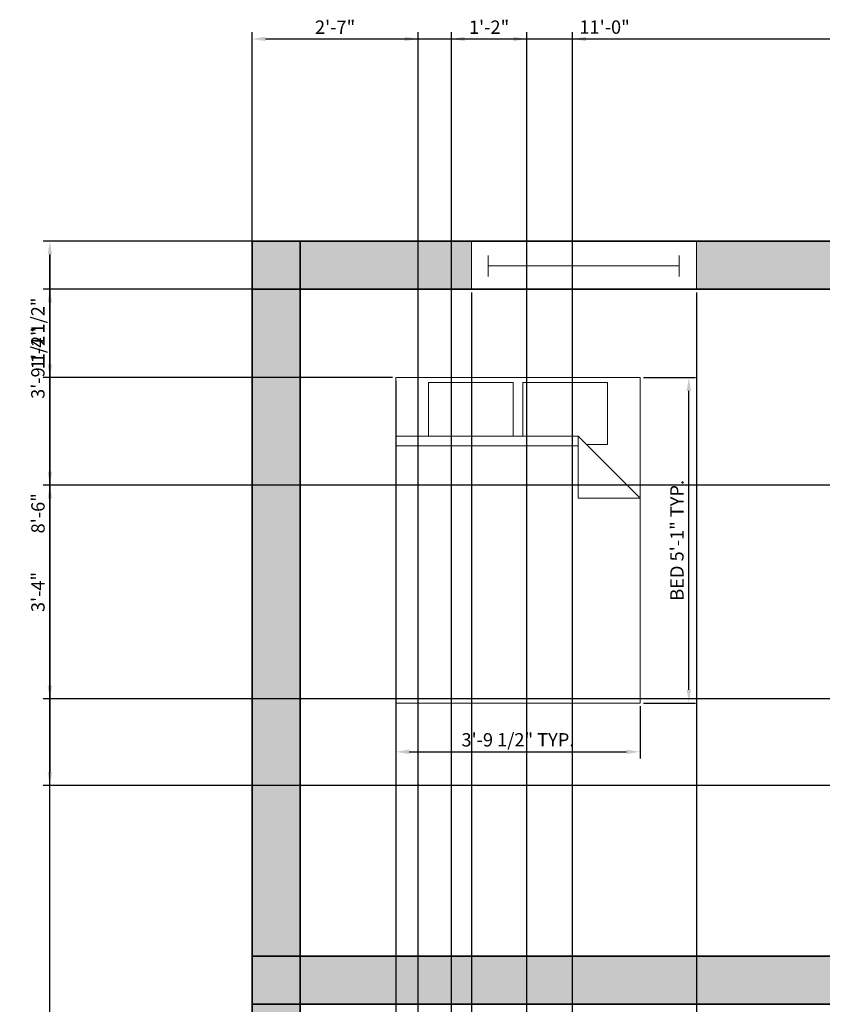
# Model space of a CAD drawing. Units: millimetres. Extents: x 2856 to 3283, y 634 to 1474.
# Tile 4 of 8: x 2856 to 3006, y 1288 to 1472. Entities that reach past the tile are written whole.
import ezdxf

# ---------------------------------------------------------------- set-up
doc = ezdxf.new("R2010")
doc.units = ezdxf.units.MM
for name, color, linetype, lineweight in [('A-ANNO-DIMS', 90, 'Continuous', 18), ('A-WALL-PATT', 2, 'Continuous', 13), ('furniture', 140, 'Continuous', 18), ('walls', 50, 'Continuous', 35), ('windows', 30, 'Continuous', 18)]:
    doc.layers.add(name, color=color, linetype=linetype, lineweight=lineweight)
doc.styles.get("Standard").update_dxf_attribs({"font": 'arial.ttf'})
doc.dimstyles.new('ISO-25', dxfattribs={"dimtxt": 2.5, "dimasz": 2.5, "dimexe": 1.25, "dimexo": 0.625, "dimtad": 1, "dimdec": 0, "dimlunit": 3, "dimtxsty": 'Standard', "dimcen": 2.5, "dimadec": 0, "dimazin": 0, "dimtfac": 1, "dimtdec": 0, "dimtmove": 0, "dimatfit": 3, "dimfxl": 1, "dimarcsym": 0})

# ---------------------------------------------------------------- blocks, each defined once
blk = doc.blocks.new('*U5')
for p, q in [((0, 4), (0, 0)), ((36, 4), (36, 0)), ((0, 2), (36, 2))]:
    blk.add_line(p, q)
blk = doc.blocks.new('Bed - Queen')
for p, q in [((0, -80.00003), (0, 0)), ((0, 0), (59.99999, 0)), ((59.99999, 0), (59.99999, -80.00003)), ((7.99999, -1.2), (28.79998, -1.2)), ((7.99999, -14.4), (7.99999, -1.2)), ((28.79998, -1.2), (28.79998, -14.4)), ((31.19999, -1.2), (51.99999, -1.2)), ((31.19999, -14.4), (31.19999, -1.2)), ((51.99999, -1.2), (51.99999, -16.4)), ((0, -14.4), (44.8, -14.4)), ((59.99999, -29.6), (44.8, -14.4)), ((44.8, -14.4), (44.8, -29.6)), ((44.8, -16.8), (0, -16.8)), ((51.99999, -16.4), (46.79936, -16.4)), ((44.8, -29.6), (59.99999, -29.6)), ((59.99999, -80.00003), (0, -80.00003))]:
    blk.add_line(p, q)
blk = doc.blocks.new('*D16')
at = {"layer": 'A-ANNO-DIMS', "color": 0, "lineweight": -2, "transparency": 16777216}
for p, q in [((2972.43, 1405.35), (2982.2, 1405.35)), ((2980.95, 1346.89), (2980.95, 1402.85)), ((2972.43, 1344.39), (2982.2, 1344.39))]:
    blk.add_line(p, q, dxfattribs=at)
at = {"layer": 'A-ANNO-DIMS', "color": 0, "transparency": 16777216}
for points in [[(2980.53, 1402.85), (2981.36, 1402.85), (2980.95, 1405.35)], [(2980.53, 1346.89), (2981.36, 1346.89), (2980.95, 1344.39)]]:
    blk.add_solid(points, dxfattribs=at)
at = {"layer": 'Defpoints', "color": 0, "transparency": 16777216}
for p in [(2971.8, 1405.35), (2980.95, 1405.35), (2971.8, 1344.39)]:
    blk.add_point(p, dxfattribs=at)
at = {"layer": 'A-ANNO-DIMS', "color": 0, "transparency": 16777216, "insert": (2979.04, 1374.87), "char_height": 2.5, "attachment_point": 5, "rotation": 90}
blk.add_mtext('BED 5\'-1" TYP.', dxfattribs=at)
blk = doc.blocks.new('*D17')
at = {"layer": 'A-ANNO-DIMS', "color": 0, "lineweight": -2, "transparency": 16777216}
for p, q in [((2926.08, 1343.77), (2926.08, 1334)), ((2971.8, 1343.77), (2971.8, 1334)), ((2928.58, 1335.25), (2969.3, 1335.25))]:
    blk.add_line(p, q, dxfattribs=at)
at = {"layer": 'A-ANNO-DIMS', "color": 0, "transparency": 16777216}
for points in [[(2928.58, 1335.66), (2928.58, 1334.83), (2926.08, 1335.25)], [(2969.3, 1335.66), (2969.3, 1334.83), (2971.8, 1335.25)]]:
    blk.add_solid(points, dxfattribs=at)
at = {"layer": 'Defpoints', "color": 0, "transparency": 16777216}
for p in [(2926.08, 1344.39), (2971.8, 1344.39), (2971.8, 1335.25)]:
    blk.add_point(p, dxfattribs=at)
at = {"layer": 'A-ANNO-DIMS', "color": 0, "transparency": 16777216, "insert": (2948.94, 1337.17), "char_height": 2.5, "attachment_point": 5}
blk.add_mtext('3\'-9 1/2" TYP.', dxfattribs=at)
blk = doc.blocks.new('*D29')
at = {"layer": 'A-ANNO-DIMS', "color": 0, "lineweight": -2, "transparency": 16777216}
for p, q in [((2898.55, 1430.94), (2860.05, 1430.94)), ((2861.3, 676.44), (2861.3, 1428.44)), ((2898.55, 673.94), (2860.05, 673.94))]:
    blk.add_line(p, q, dxfattribs=at)
at = {"layer": 'A-ANNO-DIMS', "color": 0, "transparency": 16777216}
for points in [[(2860.88, 1428.44), (2861.72, 1428.44), (2861.3, 1430.94)], [(2860.88, 676.44), (2861.72, 676.44), (2861.3, 673.94)]]:
    blk.add_solid(points, dxfattribs=at)
at = {"layer": 'Defpoints', "color": 0, "transparency": 16777216}
for p in [(2861.3, 1430.94), (2899.17, 1430.94), (2899.17, 673.94)]:
    blk.add_point(p, dxfattribs=at)
at = {"layer": 'A-ANNO-DIMS', "color": 0, "transparency": 16777216, "insert": (2859.4, 1052.44), "char_height": 2.5, "attachment_point": 5, "rotation": 90}
blk.add_mtext('63\'-1"', dxfattribs=at)
blk = doc.blocks.new('*D44')
at = {"layer": 'A-ANNO-DIMS', "color": 0, "lineweight": -2, "transparency": 16777216}
for p, q in [((2899.17, 1431.56), (2899.17, 1470.06)), ((2901.67, 1468.81), (3028.67, 1468.81)), ((3031.17, 1431.56), (3031.17, 1470.06))]:
    blk.add_line(p, q, dxfattribs=at)
at = {"layer": 'A-ANNO-DIMS', "color": 0, "transparency": 16777216}
for points in [[(2901.67, 1469.23), (2901.67, 1468.4), (2899.17, 1468.81)], [(3028.67, 1469.23), (3028.67, 1468.4), (3031.17, 1468.81)]]:
    blk.add_solid(points, dxfattribs=at)
at = {"layer": 'Defpoints', "color": 0, "transparency": 16777216}
for p in [(3031.17, 1468.81), (2899.17, 1430.94), (3031.17, 1430.94)]:
    blk.add_point(p, dxfattribs=at)
at = {"layer": 'A-ANNO-DIMS', "color": 0, "transparency": 16777216, "insert": (2965.17, 1470.71), "char_height": 2.5, "attachment_point": 5}
blk.add_mtext('11\'-0"', dxfattribs=at)
blk = doc.blocks.new('*D48')
at = {"layer": 'A-ANNO-DIMS', "color": 0, "lineweight": -2, "transparency": 16777216}
for p, q in [((3030.55, 1430.94), (2860.05, 1430.94)), ((2861.3, 1428.44), (2861.3, 1331.44)), ((3030.55, 1328.94), (2860.05, 1328.94))]:
    blk.add_line(p, q, dxfattribs=at)
at = {"layer": 'A-ANNO-DIMS', "color": 0, "transparency": 16777216}
for points in [[(2860.88, 1428.44), (2861.72, 1428.44), (2861.3, 1430.94)], [(2860.88, 1331.44), (2861.72, 1331.44), (2861.3, 1328.94)]]:
    blk.add_solid(points, dxfattribs=at)
at = {"layer": 'Defpoints', "color": 0, "transparency": 16777216}
for p in [(3031.17, 1430.94), (2861.3, 1328.94), (3031.17, 1328.94)]:
    blk.add_point(p, dxfattribs=at)
at = {"layer": 'A-ANNO-DIMS', "color": 0, "transparency": 16777216, "insert": (2859.4, 1379.94), "char_height": 2.5, "attachment_point": 5, "rotation": 90}
blk.add_mtext('8\'-6"', dxfattribs=at)
blk = doc.blocks.new('*D59')
at = {"layer": 'A-ANNO-DIMS', "color": 0, "lineweight": -2, "transparency": 16777216}
for p, q in [((2959.17, 1117.56), (2959.17, 1470.06)), ((2961.67, 1468.81), (3071.67, 1468.81)), ((3074.17, 1117.56), (3074.17, 1470.06))]:
    blk.add_line(p, q, dxfattribs=at)
at = {"layer": 'A-ANNO-DIMS', "color": 0, "transparency": 16777216}
for points in [[(2961.67, 1469.23), (2961.67, 1468.4), (2959.17, 1468.81)], [(3071.67, 1469.23), (3071.67, 1468.4), (3074.17, 1468.81)]]:
    blk.add_solid(points, dxfattribs=at)
at = {"layer": 'Defpoints', "color": 0, "transparency": 16777216}
for p in [(3074.17, 1468.81), (2959.17, 1116.94), (3074.17, 1116.94)]:
    blk.add_point(p, dxfattribs=at)
at = {"layer": 'A-ANNO-DIMS', "color": 0, "transparency": 16777216, "insert": (3016.67, 1470.71), "char_height": 2.5, "attachment_point": 5}
blk.add_mtext('9\'-7"', dxfattribs=at)
blk = doc.blocks.new('*D69')
at = {"layer": 'A-ANNO-DIMS', "color": 0, "lineweight": -2, "transparency": 16777216}
for p, q in [((2940.27, 1421.31), (2940.27, 634.81)), ((2982.35, 1421.31), (2982.35, 634.81)), ((2942.77, 636.06), (2979.85, 636.06))]:
    blk.add_line(p, q, dxfattribs=at)
at = {"layer": 'A-ANNO-DIMS', "color": 0, "transparency": 16777216}
for points in [[(2942.77, 636.48), (2942.77, 635.65), (2940.27, 636.06)], [(2979.85, 636.48), (2979.85, 635.65), (2982.35, 636.06)]]:
    blk.add_solid(points, dxfattribs=at)
at = {"layer": 'Defpoints', "color": 0, "transparency": 16777216}
for p in [(2940.27, 1421.94), (2982.35, 1421.94), (2982.35, 636.06)]:
    blk.add_point(p, dxfattribs=at)
at = {"layer": 'A-ANNO-DIMS', "color": 0, "transparency": 16777216, "insert": (2961.31, 637.97), "char_height": 2.5, "attachment_point": 5}
blk.add_mtext('3\'-6"', dxfattribs=at)
blk = doc.blocks.new('*D72')
at = {"layer": 'A-ANNO-DIMS', "color": 0, "lineweight": -2, "transparency": 16777216}
for p, q in [((3233.55, 1385.21), (2860.05, 1385.21)), ((2861.3, 1347.66), (2861.3, 1382.71)), ((3233.55, 1345.16), (2860.05, 1345.16))]:
    blk.add_line(p, q, dxfattribs=at)
at = {"layer": 'A-ANNO-DIMS', "color": 0, "transparency": 16777216}
for points in [[(2860.88, 1382.71), (2861.72, 1382.71), (2861.3, 1385.21)], [(2860.88, 1347.66), (2861.72, 1347.66), (2861.3, 1345.16)]]:
    blk.add_solid(points, dxfattribs=at)
at = {"layer": 'Defpoints', "color": 0, "transparency": 16777216}
for p in [(2861.3, 1385.21), (3234.17, 1385.21), (3234.17, 1345.16)]:
    blk.add_point(p, dxfattribs=at)
at = {"layer": 'A-ANNO-DIMS', "color": 0, "transparency": 16777216, "insert": (2859.4, 1365.19), "char_height": 2.5, "attachment_point": 5, "rotation": 90}
blk.add_mtext('3\'-4"', dxfattribs=at)
blk = doc.blocks.new('*D76')
at = {"layer": 'A-ANNO-DIMS', "color": 0, "lineweight": -2, "transparency": 16777216}
for p, q in [((2899.17, 1421.31), (2899.17, 634.81)), ((2940.27, 1421.31), (2940.27, 634.81)), ((2901.67, 636.06), (2937.77, 636.06))]:
    blk.add_line(p, q, dxfattribs=at)
at = {"layer": 'A-ANNO-DIMS', "color": 0, "transparency": 16777216}
for points in [[(2901.67, 636.48), (2901.67, 635.65), (2899.17, 636.06)], [(2937.77, 636.48), (2937.77, 635.65), (2940.27, 636.06)]]:
    blk.add_solid(points, dxfattribs=at)
at = {"layer": 'Defpoints', "color": 0, "transparency": 16777216}
for p in [(2899.17, 1421.94), (2940.27, 1421.94), (2940.27, 636.06)]:
    blk.add_point(p, dxfattribs=at)
at = {"layer": 'A-ANNO-DIMS', "color": 0, "transparency": 16777216, "insert": (2919.72, 637.97), "char_height": 2.5, "attachment_point": 5}
blk.add_mtext('3\'-5"', dxfattribs=at)
blk = doc.blocks.new('*D78')
at = {"layer": 'A-ANNO-DIMS', "color": 0, "lineweight": -2, "transparency": 16777216}
for p, q in [((3233.55, 1430.94), (2860.05, 1430.94)), ((2861.3, 1387.71), (2861.3, 1428.44)), ((3233.55, 1385.21), (2860.05, 1385.21))]:
    blk.add_line(p, q, dxfattribs=at)
at = {"layer": 'A-ANNO-DIMS', "color": 0, "transparency": 16777216}
for points in [[(2860.88, 1428.44), (2861.72, 1428.44), (2861.3, 1430.94)], [(2860.88, 1387.71), (2861.72, 1387.71), (2861.3, 1385.21)]]:
    blk.add_solid(points, dxfattribs=at)
at = {"layer": 'Defpoints', "color": 0, "transparency": 16777216}
for p in [(2861.3, 1430.94), (3234.17, 1430.94), (3234.17, 1385.21)]:
    blk.add_point(p, dxfattribs=at)
at = {"layer": 'A-ANNO-DIMS', "color": 0, "transparency": 16777216, "insert": (2859.38, 1408.08), "char_height": 2.5, "attachment_point": 5, "rotation": 90}
blk.add_mtext('3\'-9 1/2"', dxfattribs=at)
blk = doc.blocks.new('*D82')
at = {"layer": 'A-ANNO-DIMS', "color": 0, "lineweight": -2, "transparency": 16777216}
for p, q in [((2936.5, 1173.36), (2936.5, 1470.06)), ((2939, 1468.81), (2948.08, 1468.81)), ((2950.58, 1173.36), (2950.58, 1470.06))]:
    blk.add_line(p, q, dxfattribs=at)
at = {"layer": 'A-ANNO-DIMS', "color": 0, "transparency": 16777216}
for points in [[(2939, 1469.23), (2939, 1468.4), (2936.5, 1468.81)], [(2948.08, 1469.23), (2948.08, 1468.4), (2950.58, 1468.81)]]:
    blk.add_solid(points, dxfattribs=at)
at = {"layer": 'Defpoints', "color": 0, "transparency": 16777216}
for p in [(2950.58, 1468.81), (2936.5, 1172.73), (2950.58, 1172.73)]:
    blk.add_point(p, dxfattribs=at)
at = {"layer": 'A-ANNO-DIMS', "color": 0, "transparency": 16777216, "insert": (2943.54, 1470.69), "char_height": 2.5, "attachment_point": 5}
blk.add_mtext('1\'-2"', dxfattribs=at)
blk = doc.blocks.new('*D86')
at = {"layer": 'A-ANNO-DIMS', "color": 0, "lineweight": -2, "transparency": 16777216}
for p, q in [((2899.17, 1059.56), (2899.17, 1470.06)), ((2901.67, 1468.81), (2927.75, 1468.81)), ((2930.25, 1059.56), (2930.25, 1470.06))]:
    blk.add_line(p, q, dxfattribs=at)
at = {"layer": 'A-ANNO-DIMS', "color": 0, "transparency": 16777216}
for points in [[(2901.67, 1469.23), (2901.67, 1468.4), (2899.17, 1468.81)], [(2927.75, 1469.23), (2927.75, 1468.4), (2930.25, 1468.81)]]:
    blk.add_solid(points, dxfattribs=at)
at = {"layer": 'Defpoints', "color": 0, "transparency": 16777216}
for p in [(2930.25, 1468.81), (2899.17, 1058.94), (2930.25, 1058.94)]:
    blk.add_point(p, dxfattribs=at)
at = {"layer": 'A-ANNO-DIMS', "color": 0, "transparency": 16777216, "insert": (2914.71, 1470.69), "char_height": 2.5, "attachment_point": 5}
blk.add_mtext('2\'-7"', dxfattribs=at)
blk = doc.blocks.new('*D90')
at = {"layer": 'A-ANNO-DIMS', "color": 0, "lineweight": -2, "transparency": 16777216}
for p, q in [((2899.17, 1421.31), (2899.17, 634.81)), ((2926.08, 1404.73), (2926.08, 634.81)), ((2901.67, 636.06), (2923.58, 636.06))]:
    blk.add_line(p, q, dxfattribs=at)
at = {"layer": 'A-ANNO-DIMS', "color": 0, "transparency": 16777216}
for points in [[(2901.67, 636.48), (2901.67, 635.65), (2899.17, 636.06)], [(2923.58, 636.48), (2923.58, 635.65), (2926.08, 636.06)]]:
    blk.add_solid(points, dxfattribs=at)
at = {"layer": 'Defpoints', "color": 0, "transparency": 16777216}
for p in [(2899.17, 1421.94), (2926.08, 1405.35), (2926.08, 636.06)]:
    blk.add_point(p, dxfattribs=at)
at = {"layer": 'A-ANNO-DIMS', "color": 0, "transparency": 16777216, "insert": (2912.63, 637.97), "char_height": 2.5, "attachment_point": 5}
blk.add_mtext('2\'-3"', dxfattribs=at)
blk = doc.blocks.new('*D91')
at = {"layer": 'A-ANNO-DIMS', "color": 0, "lineweight": -2, "transparency": 16777216}
for p, q in [((2939.65, 1421.94), (2860.05, 1421.94)), ((2861.3, 1419.44), (2861.3, 1407.85)), ((2925.46, 1405.35), (2860.05, 1405.35))]:
    blk.add_line(p, q, dxfattribs=at)
at = {"layer": 'A-ANNO-DIMS', "color": 0, "transparency": 16777216}
for points in [[(2860.88, 1419.44), (2861.72, 1419.44), (2861.3, 1421.94)], [(2860.88, 1407.85), (2861.72, 1407.85), (2861.3, 1405.35)]]:
    blk.add_solid(points, dxfattribs=at)
at = {"layer": 'Defpoints', "color": 0, "transparency": 16777216}
for p in [(2940.27, 1421.94), (2861.3, 1405.35), (2926.08, 1405.35)]:
    blk.add_point(p, dxfattribs=at)
at = {"layer": 'A-ANNO-DIMS', "color": 0, "transparency": 16777216, "insert": (2859.38, 1413.65), "char_height": 2.5, "attachment_point": 5, "rotation": 90}
blk.add_mtext('1\'-4 1/2"', dxfattribs=at)

msp = doc.modelspace()

# ---------------------------------------------------------------- hatches: boundary and pattern name
at = {"layer": 'A-WALL-PATT'}
h = msp.add_hatch(color=256, dxfattribs=at)
h.dxf.hatch_style = 1
h.paths.add_polyline_path([(2908.17, 1430.94), (2899.17, 1430.94), (2899.17, 1421.94), (2908.17, 1421.94)])
h.paths.add_polyline_path([(2908.17, 1421.94), (2899.17, 1421.94), (2899.17, 1296.94), (2908.17, 1296.94)])
h.paths.add_polyline_path([(2940.27, 1430.94), (2908.17, 1430.94), (2908.17, 1421.94), (2940.27, 1421.94)])
h.paths.add_polyline_path([(3031.17, 1430.94), (2982.35, 1430.94), (2982.35, 1421.94), (3031.17, 1421.94)])
h.paths.add_polyline_path([(3150.5, 1430.94), (3097.17, 1430.94), (3097.17, 1421.94), (3150.5, 1421.94)])
h.paths.add_polyline_path([(3097.17, 1430.94), (3088.17, 1430.94), (3088.17, 1421.94), (3097.17, 1421.94)])
h.paths.add_polyline_path([(3097.17, 1421.94), (3088.17, 1421.94), (3088.17, 1337.94), (3097.17, 1337.94)])
h.paths.add_polyline_path([(3088.17, 1337.94), (3040.17, 1337.94), (3040.17, 1328.94), (3088.17, 1328.94)])
h.paths.add_polyline_path([(3097.17, 1337.94), (3088.17, 1337.94), (3088.17, 1328.94), (3097.17, 1328.94)])
h.paths.add_polyline_path([(3097.17, 1328.94), (3088.17, 1328.94), (3088.17, 1296.94), (3097.17, 1296.94)])
h.paths.add_polyline_path([(3097.17, 1296.94), (3088.17, 1296.94), (3088.17, 1287.94), (3097.17, 1287.94)])
h.paths.add_polyline_path([(3040.17, 1421.94), (3031.17, 1421.94), (3031.17, 1337.94), (3040.17, 1337.94)])
h.paths.add_polyline_path([(3040.17, 1337.94), (3031.17, 1337.94), (3031.17, 1328.94), (3040.17, 1328.94)])
h.paths.add_polyline_path([(3040.17, 1430.94), (3031.17, 1430.94), (3031.17, 1421.94), (3040.17, 1421.94)])
h.paths.add_polyline_path([(3243.17, 1421.94), (3234.17, 1421.94), (3234.17, 1385.21), (3243.17, 1385.21)])
h.paths.add_polyline_path([(3243.17, 1430.94), (3234.17, 1430.94), (3234.17, 1421.94), (3243.17, 1421.94)])
h.paths.add_polyline_path([(3234.17, 1430.94), (3189.65, 1430.94), (3189.65, 1421.94), (3234.17, 1421.94)])
h.paths.add_polyline_path([(3243.17, 1345.16), (3234.17, 1345.16), (3234.17, 1296.94), (3243.17, 1296.94)])
h.paths.add_polyline_path([(3234.17, 1296.94), (3128.45, 1296.94, -0.06768), (3129.44, 1289.59), (3129.44, 1287.94), (3234.17, 1287.94)])
h.paths.add_polyline_path([(3031.17, 1296.94), (2908.17, 1296.94), (2908.17, 1287.94), (3031.17, 1287.94)])
h.paths.add_polyline_path([(3040.17, 1296.94), (3031.17, 1296.94), (3031.17, 1287.94), (3040.17, 1287.94)])
h.paths.add_polyline_path([(2908.17, 1296.94), (2899.17, 1296.94), (2899.17, 1287.94), (2908.17, 1287.94)])
h.paths.add_polyline_path([(2908.17, 1287.94), (2899.17, 1287.94), (2899.17, 1235.12), (2908.17, 1235.12)])
h.paths.add_polyline_path([(3040.17, 1287.94), (3031.17, 1287.94), (3031.17, 1165.94), (3040.17, 1165.94)])
h.paths.add_polyline_path([(3165.17, 1165.94), (3040.17, 1165.94), (3040.17, 1156.94), (3165.17, 1156.94)])
h.paths.add_polyline_path([(3040.17, 1165.94), (3031.17, 1165.94), (3031.17, 1156.94), (3040.17, 1156.94)])
h.paths.add_polyline_path([(3040.17, 1156.94), (3031.17, 1156.94), (3031.17, 1147.75, -0.068303), (3038.59, 1148.77), (3040.17, 1148.77)])
h.paths.add_polyline_path([(3174.17, 1197.55), (3166.11, 1197.55), (3165.17, 1197.55), (3165.17, 1165.94), (3174.17, 1165.94)])
h.paths.add_polyline_path([(3174.17, 1165.94), (3165.17, 1165.94), (3165.17, 1156.94), (3174.17, 1156.94)])
h.paths.add_polyline_path([(3234.17, 1165.94), (3174.17, 1165.94), (3174.17, 1156.94), (3234.17, 1156.94)])
h.paths.add_polyline_path([(3243.17, 1165.94), (3234.17, 1165.94), (3234.17, 1156.94), (3243.17, 1156.94)])
h.paths.add_polyline_path([(3243.17, 1172.31), (3234.17, 1172.31), (3234.17, 1165.94), (3243.17, 1165.94)])
h.paths.add_polyline_path([(3243.17, 1222.94), (3234.17, 1222.94), (3234.17, 1213.94), (3243.17, 1213.94)])
h.paths.add_polyline_path([(3234.17, 1222.94), (3174.17, 1222.94), (3174.17, 1213.94), (3234.17, 1213.94)])
h.paths.add_polyline_path([(3174.17, 1222.94), (3165.17, 1222.94), (3165.17, 1213.94), (3174.17, 1213.94)])
h.paths.add_polyline_path([(3174.17, 1270.54, -0.139319), (3166.75, 1268.43), (3165.17, 1268.43), (3165.17, 1222.94), (3174.17, 1222.94)])
h.paths.add_polyline_path([(3243.17, 1243.94), (3234.17, 1243.94), (3234.17, 1222.94), (3243.17, 1222.94)])
h.paths.add_polyline_path([(3243.17, 1213.94), (3234.17, 1213.94), (3234.17, 1203.68), (3243.17, 1203.68)])
h.paths.add_polyline_path([(3174.17, 1213.94), (3165.17, 1213.94), (3165.17, 1210.62), (3166.11, 1210.62, -0.16772), (3174.17, 1207.84)])
h.paths.add_polyline_path([(3243.17, 1296.94), (3234.17, 1296.94), (3234.17, 1287.94), (3243.17, 1287.94)])
h.paths.add_polyline_path([(3243.17, 1287.94), (3234.17, 1287.94), (3234.17, 1276.76), (3243.17, 1276.76)])
h.paths.add_polyline_path([(3174.17, 1287.94), (3165.17, 1287.94), (3165.17, 1282.56), (3166.75, 1282.56), (3174.17, 1282.56)])
h.paths.add_polyline_path([(2908.17, 1190.69), (2899.17, 1190.69), (2899.17, 1116.94), (2908.17, 1116.94)])
h.paths.add_polyline_path([(2908.17, 1107.94), (2899.17, 1107.94), (2899.17, 1058.94), (2908.17, 1058.94)])
h.paths.add_polyline_path([(2908.17, 1116.94), (2899.17, 1116.94), (2899.17, 1107.94), (2908.17, 1107.94)])
h.paths.add_polyline_path([(2959.17, 1107.94), (2950.17, 1107.94), (2950.17, 1058.94), (2959.17, 1058.94)])
h.paths.add_polyline_path([(2959.17, 1116.94), (2950.17, 1116.94), (2950.17, 1107.94), (2959.17, 1107.94)])
h.paths.add_polyline_path([(2950.17, 1116.94), (2908.17, 1116.94), (2908.17, 1107.94), (2950.17, 1107.94)])
h.paths.add_polyline_path([(3031.17, 1116.94), (2959.17, 1116.94), (2959.17, 1107.94), (3031.17, 1107.94)])
h.paths.add_polyline_path([(3074.17, 1116.94), (3065.17, 1116.94), (3065.17, 1107.94), (3074.17, 1107.94)])
h.paths.add_polyline_path([(3065.17, 1116.94), (3040.17, 1116.94), (3040.17, 1107.94), (3065.17, 1107.94)])
h.paths.add_polyline_path([(3040.17, 1116.94), (3031.17, 1116.94), (3031.17, 1107.94), (3040.17, 1107.94)])
h.paths.add_polyline_path([(3040.17, 1121.26), (3038.59, 1121.26), (3031.17, 1121.26), (3031.17, 1116.94), (3040.17, 1116.94)])
h.paths.add_polyline_path([(3074.17, 1107.94), (3065.17, 1107.94), (3065.17, 1058.94), (3074.17, 1058.94)])
h.paths.add_polyline_path([(3074.17, 1058.94), (3065.17, 1058.94), (3065.17, 1049.94), (3074.17, 1049.94)])
h.paths.add_polyline_path([(3065.17, 1058.94), (2975.4, 1058.94, -0.174756), (2978.69, 1049.94), (3065.17, 1049.94)])
h.paths.add_polyline_path([(2929.83, 1051.89), (2930.25, 1058.94), (2908.17, 1058.94), (2908.17, 1049.94), (2929.71, 1049.94)])
h.paths.add_polyline_path([(2908.17, 1058.94), (2899.17, 1058.94), (2899.17, 1049.94), (2908.17, 1049.94)])
h.paths.add_polyline_path([(2950.17, 1058.94), (2942.07, 1058.94, -0.146602), (2943.93, 1051.05), (2943.86, 1049.94), (2950.17, 1049.94)])
h.paths.add_polyline_path([(2959.17, 1058.94), (2950.17, 1058.94), (2950.17, 1049.94), (2959.17, 1049.94)])
h.paths.add_polyline_path([(2964.56, 1058.94), (2959.17, 1058.94), (2959.17, 1049.94), (2964.56, 1049.94)])
h.paths.add_polyline_path([(2908.17, 1049.94), (2899.17, 1049.94), (2899.17, 799.94), (2908.17, 799.94)])
h.paths.add_polyline_path([(3234.17, 1058.94), (3074.17, 1058.94), (3074.17, 1049.94), (3234.17, 1049.94)])
h.paths.add_polyline_path([(3243.17, 1156.94), (3234.17, 1156.94), (3234.17, 1058.94), (3243.17, 1058.94)])
h.paths.add_polyline_path([(3243.17, 1058.94), (3234.17, 1058.94), (3234.17, 1049.94), (3243.17, 1049.94)])
h.paths.add_polyline_path([(3243.17, 1049.94), (3234.17, 1049.94), (3234.17, 931.7), (3234.17, 799.94), (3243.17, 799.94), (3243.17, 931.7)])
h.paths.add_polyline_path([(2908.17, 790.94), (2899.17, 790.94), (2899.17, 682.94), (2908.17, 682.94)])
h.paths.add_polyline_path([(2908.17, 799.94), (2899.17, 799.94), (2899.17, 790.94), (2908.17, 790.94)])
h.paths.add_polyline_path([(3234.17, 799.94), (2908.17, 799.94), (2908.17, 790.94), (3234.17, 790.94)])
h.paths.add_polyline_path([(3243.17, 799.94), (3234.17, 799.94), (3234.17, 790.94), (3243.17, 790.94)])
h.paths.add_polyline_path([(3243.17, 790.94), (3234.17, 790.94), (3234.17, 682.94), (3243.17, 682.94)])
h.paths.add_polyline_path([(3234.17, 682.94), (2908.17, 682.94), (2908.17, 673.94), (3234.17, 673.94)])
h.paths.add_polyline_path([(3243.17, 682.94), (3234.17, 682.94), (3234.17, 673.94), (3243.17, 673.94)])
h.paths.add_polyline_path([(2908.17, 682.94), (2899.17, 682.94), (2899.17, 673.94), (2908.17, 673.94)])

# ---------------------------------------------------------------- linework, layer by layer
at = {"layer": 'walls'}
for p, q in [((2899.17, 1430.94), (2899.17, 790.94)), ((2899.17, 1430.94), (3243.17, 1430.94)), ((2908.17, 1430.94), (2908.17, 790.94)), ((2899.17, 1421.94), (3243.17, 1421.94)), ((2899.17, 1296.94), (3040.17, 1296.94)), ((2899.17, 1296.94), (3040.17, 1296.94)), ((2899.17, 1287.94), (3040.17, 1287.94)), ((2899.17, 1287.94), (3040.17, 1287.94))]:
    msp.add_line(p, q, dxfattribs=at)
at = {"layer": 'windows'}
for p, q in [((2940.27, 1421.94), (2940.27, 1430.94)), ((2982.35, 1421.94), (2982.35, 1430.94))]:
    msp.add_line(p, q, dxfattribs=at)

# ---------------------------------------------------------------- block references
at = {"layer": 'furniture', "xscale": 0.7619997142501188, "yscale": 0.7619997142501188, "zscale": 0.7619997142501188}
msp.add_blockref('Bed - Queen', (2926.08, 1405.35), dxfattribs=at)
at = {"layer": 'windows', "xscale": 0.9925939517092485, "yscale": 0.9925939517092485, "zscale": 0.9925939517092485}
msp.add_blockref('*U5', (2943.4, 1424.29), dxfattribs=at)

# ---------------------------------------------------------------- dimensions: what is measured, and where the dimension line sits
at = {"layer": 'A-ANNO-DIMS'}
for base, p1, p2, picture, middle in [((3031.17, 1468.81), (2899.17, 1430.94), (3031.17, 1430.94), '*D44', (2965.17, 1470.71)), ((2930.25, 1468.81), (2899.17, 1058.94), (2930.25, 1058.94), '*D86', (2914.71, 1470.69)), ((2950.58, 1468.81), (2936.5, 1172.73), (2950.58, 1172.73), '*D82', (2943.54, 1470.69)), ((3074.17, 1468.81), (2959.17, 1116.94), (3074.17, 1116.94), '*D59', (3016.67, 1470.71)), ((2940.27, 636.06), (2899.17, 1421.94), (2940.27, 1421.94), '*D76', (2919.72, 637.97)), ((2926.08, 636.06), (2899.17, 1421.94), (2926.08, 1405.35), '*D90', (2912.63, 637.97)), ((2982.35, 636.06), (2940.27, 1421.94), (2982.35, 1421.94), '*D69', (2961.31, 637.97))]:
    dim = msp.add_linear_dim(base=base, p1=p1, p2=p2, dimstyle='ISO-25', override={"dimdec": 1, "dimlfac": 1, "dimrnd": 0, "dimzin": 1, "dimdsep": 46, "dimlunit": 4, "dimfrac": 2}, dxfattribs=at)
    dim.commit()
    dim.dimension.update_dxf_attribs({"geometry": picture, "text_midpoint": middle})
for base, p1, p2, picture, middle in [((2861.3, 1430.94), (3234.17, 1385.21), (3234.17, 1430.94), '*D78', (2859.38, 1408.08)), ((2861.3, 1430.94), (2899.17, 673.94), (2899.17, 1430.94), '*D29', (2859.4, 1052.44)), ((2861.3, 1328.94), (3031.17, 1430.94), (3031.17, 1328.94), '*D48', (2859.4, 1379.94)), ((2861.3, 1405.35), (2940.27, 1421.94), (2926.08, 1405.35), '*D91', (2859.38, 1413.65)), ((2861.3003, 1385.2147), (3234.1743, 1345.1601), (3234.1743, 1385.2147), '*D72', (2859.3981, 1365.1874))]:
    dim = msp.add_linear_dim(base=base, p1=p1, p2=p2, angle=90, dimstyle='ISO-25', override={"dimdec": 1, "dimlfac": 1, "dimrnd": 0, "dimzin": 1, "dimdsep": 46, "dimlunit": 4, "dimfrac": 2}, dxfattribs=at)
    dim.commit()
    dim.dimension.update_dxf_attribs({"geometry": picture, "text_midpoint": middle})
dim = msp.add_linear_dim(base=(2980.95, 1405.35), p1=(2971.8, 1344.39), p2=(2971.8, 1405.35), angle=90, text='BED <> TYP.', dimstyle='ISO-25', override={"dimdec": 1, "dimlfac": 1, "dimrnd": 0, "dimzin": 1, "dimdsep": 46, "dimlunit": 4, "dimfrac": 2}, dxfattribs=at)
dim.commit()
dim.dimension.update_dxf_attribs({"geometry": '*D16', "text_midpoint": (2979.04, 1374.87)})
dim = msp.add_linear_dim(base=(2971.8, 1335.25), p1=(2926.08, 1344.39), p2=(2971.8, 1344.39), text='<> TYP.', dimstyle='ISO-25', override={"dimdec": 1, "dimlfac": 1, "dimrnd": 0, "dimzin": 1, "dimdsep": 46, "dimlunit": 4, "dimfrac": 2}, dxfattribs=at)
dim.commit()
dim.dimension.update_dxf_attribs({"geometry": '*D17', "text_midpoint": (2948.94, 1337.17)})

doc.saveas('drawing.dxf')
